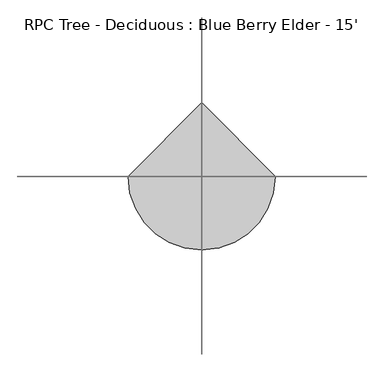
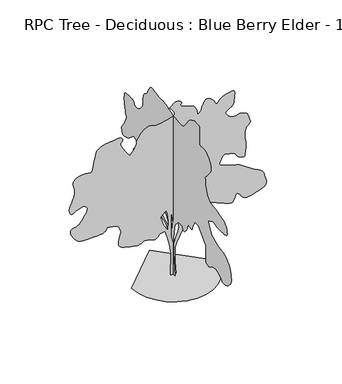
"""IFC4 building model written with IfcOpenShell, lengths in millimetres: geographic element geometry, RPC Tree - Deciduous : Blue Berry Elder - 15'."""

from ifc_helpers import new_model, si_unit, origin, place, context, project, spatial, triangles, source, transform, mapped, element, save


def rpc_tree_deciduous_blue_berry_elder_15_a2d70376(model_context):
    return source(origin(), model_context, "Body", "Tessellation", [
        triangles([(-0.0014919, 59.6430573, 0.0042007), (-0.0014919, -63.4980182, 0.0042007), (-0.0014919, -15.6099892, 574.662743), (-0.0014919, -1.9275415, 923.5625221), (-0.0014919, -22.4510529, 1121.9570257), (-0.0014919, -77.1804997, 1347.7149754), (-0.0014919, -227.6865383, 1498.2227943), (-0.0014919, -385.0338381, 1498.2227943), (-0.0014919, -419.2400351, 1402.4443382), (-0.0014919, -487.6499219, 1409.2870892), (-0.0014919, -562.9051031, 1498.2227943), (-0.0014919, -610.791715, 1593.9986343), (-0.0014919, -638.1577045, 1689.7744743), (-0.0014919, -713.4103786, 1662.4110283), (-0.0014919, -795.5032602, 1655.5682774), (-0.0014919, -870.7558617, 1826.5992622), (-0.0014919, -925.4852972, 1929.2153824), (-0.0014919, -1075.9931162, 1922.3751022), (-0.0014919, -1192.2921947, 1826.5992622), (-0.0014919, -1404.3696568, 1600.8387691), (-0.0014919, -1411.2099369, 1375.0808922), (-0.0014919, -1409.1144253, 1348.2534599), (-0.0014919, -1404.5093285, 1316.2824463), (-0.0014919, -1399.9017609, 1281.557967), (-0.0014919, -1397.8062492, 1246.4730446), (-0.0014919, -1400.7374657, 1213.4249891), (-0.0014919, -1411.2099369, 1184.8042797), (-0.0014919, -1431.7331028, 1163.0034302), (-0.0014919, -1457.4226685, 1147.2477785), (-0.0014919, -1482.2740585, 1135.79746), (-0.0014919, -1507.1254486, 1129.6151339), (-0.0014919, -1532.8150143, 1129.6557564), (-0.0014919, -1560.1810764, 1136.8769726), (-0.0014919, -1590.0565784, 1152.2338114), (-0.0014919, -1623.2873989, 1176.6863886), (-0.0014919, -1664.49375, 1202.6350954), (-0.0014919, -1715.0347057, 1221.7613262), (-0.0014919, -1770.8411831, 1233.9482277), (-0.0014919, -1827.8439537, 1239.0739323), (-0.0014919, -1881.9739346, 1237.0215866), (-0.0014919, -1929.1645134, 1227.6667797), (-0.0014919, -1965.3442818, 1210.8926582), (-0.0014919, -1995.2630951, 1185.7212296), (-0.0014919, -2027.0942917, 1154.4487198), (-0.0014919, -2061.9177475, 1121.8579039), (-0.0014919, -2100.8127571, 1092.7367889), (-0.0014919, -2144.8513481, 1071.8757803), (-0.0014919, -2195.1129604, 1064.0551094), (-0.0014919, -2252.6744179, 1074.0677977), (-0.0014919, -2311.551638, 1100.7352833), (-0.0014919, -2364.3279224, 1137.4535362), (-0.0014919, -2409.9209244, 1180.8748684), (-0.0014919, -2447.2590523, 1227.6464321), (-0.0014919, -2475.2625755, 1274.4181412), (-0.0014919, -2492.8519089, 1317.8368572), (-0.0014919, -2498.9556061, 1354.5577263), (-0.0014919, -2495.0465424, 1394.6871082), (-0.0014919, -2484.4370155, 1446.9019444), (-0.0014919, -2468.7981445, 1505.7005356), (-0.0014919, -2449.8115128, 1565.5759506), (-0.0014919, -2429.1486752, 1621.024165), (-0.0014919, -2408.4858376, 1666.538538), (-0.0014919, -2389.496735, 1696.6146091), (-0.0014919, -2367.4393604, 1721.5473896), (-0.0014919, -2337.0025555, 1752.8198994), (-0.0014919, -2299.0269665, 1786.7288761), (-0.0014919, -2254.3509144, 1819.5584129), (-0.0014919, -2203.8099586, 1847.6000153), (-0.0014919, -2148.2422749, 1867.1453339), (-0.0014919, -2088.4861839, 1874.4858742), (-0.0014919, -2026.3171589, 1879.471907), (-0.0014919, -1963.0710194, 1893.4344269), (-0.0014919, -1898.9284229, 1914.8745426), (-0.0014919, -1834.0668297, 1942.2988861), (-0.0014919, -1768.6668972, 1974.2114731), (-0.0014919, -1702.9062309, 2009.1161739), (-0.0014919, -1636.9678139, 2045.5143883), (-0.0014919, -1493.3027458, 2312.3213585), (-0.0014919, -1712.220488, 2414.9399494), (-0.0014919, -1741.6996479, 2406.2024014), (-0.0014919, -1772.1365982, 2397.8254417), (-0.0014919, -1804.4885479, 2390.1673336), (-0.0014919, -1839.7108166, 2383.5861946), (-0.0014919, -1878.7633747, 2378.4401424), (-0.0014919, -1922.603722, 2375.0899109), (-0.0014919, -1972.187178, 2373.8910015), (-0.0014919, -2028.8316856, 2373.6725555), (-0.0014919, -2090.261657, 2373.8122272), (-0.0014919, -2152.0522167, 2375.5064552), (-0.0014919, -2209.7738388, 2379.9564743), (-0.0014919, -2258.9965611, 2388.3511654), (-0.0014919, -2295.2982697, 2401.8945248), (-0.0014919, -2314.2440609, 2421.7802296), (-0.0014919, -2317.876252, 2453.1136368), (-0.0014919, -2312.2908371, 2496.5351143), (-0.0014919, -2299.1666382, 2546.5297371), (-0.0014919, -2280.1775356, 2597.6091774), (-0.0014919, -2257.0026421, 2644.26912), (-0.0014919, -2231.3130764, 2680.9974014), (-0.0014919, -2204.7853352, 2702.2574409), (-0.0014919, -2178.018655, 2712.9253944), (-0.0014919, -2148.9788578, 2722.1454712), (-0.0014919, -2115.3923904, 2730.9847572), (-0.0014919, -2074.9835197, 2740.5606262), (-0.0014919, -2025.478838, 2751.9398735), (-0.0014919, -1964.605228, 2766.1637146), (-0.0014919, -1890.091753, 2784.3501045), (-0.0014919, -1810.2315113, 2802.4350471), (-0.0014919, -1735.3979977, 2817.522789), (-0.0014919, -1666.4267715, 2832.4579239), (-0.0014919, -1604.1586246, 2850.1870743), (-0.0014919, -1549.4291164, 2873.5298355), (-0.0014919, -1503.0767132, 2905.3557999), (-0.0014919, -1465.9392998, 2948.5613022), (-0.0014919, -1437.478537, 3000.783696), (-0.0014919, -1415.8377068, 3057.3241402), (-0.0014919, -1399.8814133, 3117.4716316), (-0.0014919, -1388.4717899, 3180.4634262), (-0.0014919, -1380.4732956, 3245.6399712), (-0.0014919, -1374.7506798, 3312.238813), (-0.0014919, -1370.1634598, 3379.5489487), (-0.0014919, -1421.161655, 3432.3047401), (-0.0014919, -1470.3080738, 3484.9335045), (-0.0014919, -1515.7412018, 3537.3337944), (-0.0014919, -1555.6115879, 3589.3785828), (-0.0014919, -1588.0626595, 3640.9149719), (-0.0014919, -1611.2401691, 3691.8929649), (-0.0014919, -1623.2873989, 3742.1340843), (-0.0014919, -1619.2183159, 3797.684182), (-0.0014919, -1597.4378139, 3860.6506874), (-0.0014919, -1561.1766552, 3925.0397804), (-0.0014919, -1513.6685085, 3984.9076378), (-0.0014919, -1458.1415199, 4034.2345688), (-0.0014919, -1397.8265968, 4067.0258812), (-0.0014919, -1335.9572628, 4077.3383331), (-0.0014919, -1278.5939037, 4074.2649742), (-0.0014919, -1229.7292992, 4071.8773293), (-0.0014919, -1189.4804478, 4071.7755913), (-0.0014919, -1157.966601, 4075.509375), (-0.0014919, -1135.3097717, 4084.6280045), (-0.0014919, -1121.6268133, 4100.6808037), (-0.0014919, -1117.0395206, 4125.2426765), (-0.0014919, -1118.7743711, 4171.0390091), (-0.0014919, -1122.5437632, 4241.9559013), (-0.0014919, -1126.1936857, 4326.2838936), (-0.0014919, -1127.5704185, 4412.288237), (-0.0014919, -1124.5173346, 4488.2344734), (-0.0014919, -1114.885655, 4542.4125618), (-0.0014919, -1096.5163548, 4563.0627548), (-0.0014919, -1069.6304232, 4564.4597626), (-0.0014919, -1037.2377783, 4567.5331215), (-0.0014919, -1001.3780485, 4570.6067711), (-0.0014919, -964.0806158, 4572.0037788), (-0.0014919, -927.380167, 4570.0477936), (-0.0014919, -893.3136417, 4563.0627548), (-0.0014919, -863.9156542, 4549.3976006), (-0.0014919, -835.993376, 4533.1416161), (-0.0014919, -805.556571, 4518.3587975), (-0.0014919, -773.4433422, 4503.0678703), (-0.0014919, -740.4944086, 4485.3895889), (-0.0014919, -707.545475, 4463.4185463), (-0.0014919, -675.4347897, 4435.2246277), (-0.0014919, -644.9979847, 4398.877137), (-0.0014919, -614.4824055, 4355.0112099), (-0.0014919, -581.8128516, 4307.6911331), (-0.0014919, -547.3475862, 4260.1167114), (-0.0014919, -511.4446541, 4215.5397812), (-0.0014919, -474.4672963, 4177.1857269), (-0.0014919, -436.7711234, 4148.2805145), (-0.0014919, -398.7168328, 4132.075399), (-0.0014919, -359.7633602, 4126.0048393), (-0.0014919, -319.1360072, 4124.6078316), (-0.0014919, -276.8322849, 4126.6905533), (-0.0014919, -232.8521387, 4131.0338928), (-0.0014919, -187.1978941, 4136.4696075), (-0.0014919, -139.8680069, 4141.7780045), (-0.0014919, -90.8629858, 4145.7658424), (-0.0014919, -33.0220578, 4153.2081207), (-0.0014919, 35.9481419, 4167.7368851), (-0.0014919, 108.7479043, 4186.3296455), (-0.0014919, 178.0769938, 4205.989492), (-0.0014919, 236.6359921, 4223.7439316), (-0.0014919, 277.1243819, 4236.5963448), (-0.0014919, 292.2424816, 4241.523951), (-0.0014919, 300.5609782, 4244.1147812), (-0.0014919, 323.5962728, 4250.5411331), (-0.0014919, 358.4806623, 4258.7705727), (-0.0014919, 402.3388501, 4266.7462486), (-0.0014919, 452.3032422, 4272.4357269), (-0.0014919, 505.495962, 4273.8327347), (-0.0014919, 559.0493792, 4268.9051285), (-0.0014919, 618.0663437, 4267.9400711), (-0.0014919, 686.0596498, 4278.836499), (-0.0014919, 757.7613779, 4295.8293571), (-0.0014919, 827.9085497, 4313.1774261), (-0.0014919, 891.2359343, 4325.1409401), (-0.0014919, 942.4728504, 4325.9789703), (-0.0014919, 976.3615522, 4309.9517509), (-0.0014919, 999.7371603, 4282.3926773), (-0.0014919, 1022.6327831, 4252.7761711), (-0.0014919, 1044.5733044, 4221.6359207), (-0.0014919, 1065.0761953, 4189.4032951), (-0.0014919, 1083.6639416, 4156.5608231), (-0.0014919, 1099.8614994, 4123.6171944), (-0.0014919, 1113.1837967, 4091.0287766), (-0.0014919, 1129.0994677, 4063.2159393), (-0.0014919, 1151.7182178, 4042.0067688), (-0.0014919, 1178.5228317, 4023.896537), (-0.0014919, 1207.0064129, 4005.4308037), (-0.0014919, 1234.6492023, 3983.1295486), (-0.0014919, 1258.9419056, 3953.5130424), (-0.0014919, 1277.3720306, 3913.1524246), (-0.0014919, 1288.5608826, 3878.2275215), (-0.0014919, 1294.0066257, 3861.6157448), (-0.0014919, 1295.50261, 3854.8086021), (-0.0014919, 1294.8448013, 3849.3223091), (-0.0014919, 1293.8262589, 3836.6730812), (-0.0014919, 1294.245274, 3808.3265556), (-0.0014919, 1297.8953419, 3755.7995293), (-0.0014919, 1304.3392799, 3695.8046448), (-0.0014919, 1312.5765678, 3648.6365936), (-0.0014919, 1323.5645599, 3611.1208603), (-0.0014919, 1338.2635174, 3580.2090843), (-0.0014919, 1357.6310852, 3552.7770378), (-0.0014919, 1382.622147, 3525.6752037), (-0.0014919, 1414.1969639, 3495.8555122), (-0.0014919, 1450.0566936, 3466.1628479), (-0.0014919, 1486.6377457, 3441.8806091), (-0.0014919, 1522.9750626, 3423.3131378), (-0.0014919, 1558.118557, 3410.8670952), (-0.0014919, 1591.1081131, 3404.8979828), (-0.0014919, 1620.9860859, 3405.7363037), (-0.0014919, 1646.795121, 3413.7628487), (-0.0014919, 1665.9440975, 3429.5107246), (-0.0014919, 1679.3451691, 3450.9992386), (-0.0014919, 1691.3136246, 3474.7736595), (-0.0014919, 1706.1523991, 3497.354258), (-0.0014919, 1728.1716946, 3515.2613045), (-0.0014919, 1761.6793877, 3525.0403587), (-0.0014919, 1810.9833549, 3523.2114006), (-0.0014919, 1870.0002468, 3519.655513), (-0.0014919, 1927.9427856, 3522.4495285), (-0.0014919, 1982.0524189, 3525.3702805), (-0.0014919, 2029.5835293, 3522.1698944), (-0.0014919, 2067.7775642, 3506.6504929), (-0.0014919, 2093.8862904, 3472.5891998), (-0.0014919, 2105.1536259, 3413.7628487), (-0.0014919, 2107.5870529, 3355.0888138), (-0.0014919, 2108.7045719, 3318.9189285), (-0.0014919, 2108.0264156, 3295.0939293), (-0.0014919, 2105.0749969, 3273.4275192), (-0.0014919, 2099.3701126, 3243.7095657), (-0.0014919, 2090.4343208, 3195.8305115), (-0.0014919, 2077.7901798, 3119.5796425), (-0.0014919, 2061.2548519, 3041.6777115), (-0.0014919, 2043.5255562, 2988.8966309), (-0.0014919, 2028.4253151, 2951.2030014), (-0.0014919, 2019.7893597, 2918.5384254), (-0.0014919, 2021.4453632, 2880.844796), (-0.0014919, 2037.2212898, 2828.0637154), (-0.0014919, 2070.9474289, 2750.1617844), (-0.0014919, 2114.4501514, 2668.4752007), (-0.0014919, 2155.0774681, 2607.7440239), (-0.0014919, 2189.9618214, 2562.9383286), (-0.0014919, 2216.2279507, 2529.0063881), (-0.0014919, 2231.0082985, 2500.9418221), (-0.0014919, 2231.4273136, 2473.7181931), (-0.0014919, 2214.6124969, 2442.3032501), (-0.0014919, 2195.0062809, 2409.7735497), (-0.0014919, 2184.256937, 2383.1061367), (-0.0014919, 2175.300943, 2363.1416576), (-0.0014919, 2161.0794273, 2350.7159626), (-0.0014919, 2134.5339546, 2346.6672272), (-0.0014919, 2088.6004211, 2351.8336269), (-0.0014919, 2016.218066, 2367.0507214), (-0.0014919, 1937.2366951, 2396.3496597), (-0.0014919, 1873.5715405, 2438.0946407), (-0.0014919, 1821.2754593, 2484.6274109), (-0.0014919, 1776.3986927, 2528.2875366), (-0.0014919, 1734.9940979, 2561.4142937), (-0.0014919, 1693.1069744, 2576.3494286), (-0.0014919, 1646.795121, 2565.45271), (-0.0014919, 1602.1392712, 2539.6566101), (-0.0014919, 1566.8155552, 2514.9450371), (-0.0014919, 1539.2717422, 2491.129921), (-0.0014919, 1517.9509506, 2468.0336563), (-0.0014919, 1501.2961533, 2445.4757309), (-0.0014919, 1487.7527939, 2423.2762138), (-0.0014919, 1475.7666069, 2401.2569183), (-0.0014919, 1494.8139908, 2382.2881634), (-0.0014919, 1513.8006226, 2363.8605091), (-0.0014919, 1532.6702557, 2346.5072079), (-0.0014919, 1551.3570511, 2330.7719765), (-0.0014919, 1569.8076691, 2317.1879219), (-0.0014919, 1587.9584507, 2306.2990517), (-0.0014919, 1605.7486439, 2298.6383274), (-0.0014919, 1624.7173988, 2295.1686264), (-0.0014919, 1645.2405647, 2294.3304508), (-0.0014919, 1665.5250824, 2292.895364), (-0.0014919, 1683.7749859, 2287.6299877), (-0.0014919, 1698.1945999, 2275.3032692), (-0.0014919, 1706.9905746, 2252.6845917), (-0.0014919, 1708.3672348, 2216.5455185), (-0.0014919, 1703.8180939, 2176.2559719), (-0.0014919, 1696.2794552, 2141.3512711), (-0.0014919, 1686.106675, 2108.8417728), (-0.0014919, 1673.6606323, 2075.7328926), (-0.0014919, 1659.3020611, 2039.0323711), (-0.0014919, 1643.3838467, 1995.7533268), (-0.0014919, 1626.2718098, 1942.8984135), (-0.0014919, 1608.601086, 1883.4013184), (-0.0014919, 1592.1266556, 1823.7848991), (-0.0014919, 1578.8829872, 1766.4443584), (-0.0014919, 1570.9048405, 1713.7673412), (-0.0014919, 1570.2266842, 1668.1539917), (-0.0014919, 1578.8829872, 1631.9944256), (-0.0014919, 1598.9083637, 1607.6815201), (-0.0014919, 1624.6970512, 1591.4839622), (-0.0014919, 1649.4087696, 1577.8035473), (-0.0014919, 1673.2237404, 1566.2135571), (-0.0014919, 1696.320005, 1556.3023888), (-0.0014919, 1718.8777851, 1547.6460857), (-0.0014919, 1741.0774475, 1539.8279583), (-0.0014919, 1763.096743, 1532.4263752), (-0.0014919, 1786.3707584, 1542.3400143), (-0.0014919, 1808.5702755, 1550.1581417), (-0.0014919, 1828.6159996, 1553.787862), (-0.0014919, 1845.4283455, 1551.135989), (-0.0014919, 1857.9352856, 1540.1073017), (-0.0014919, 1865.0549091, 1518.6062885), (-0.0014919, 1865.7127178, 1484.5397633), (-0.0014919, 1859.7895329, 1448.2787498), (-0.0014919, 1848.4813568, 1420.635815), (-0.0014919, 1832.6850826, 1400.1710758), (-0.0014919, 1813.2973125, 1385.4517708), (-0.0014919, 1791.2171196, 1375.040197), (-0.0014919, 1767.3435768, 1367.5015583), (-0.0014919, 1742.570961, 1361.3978611), (-0.0014919, 1730.8234222, 1353.9581989), (-0.0014919, 1718.9565594, 1345.8607281), (-0.0014919, 1706.8509029, 1336.4474945), (-0.0014919, 1694.3845127, 1325.0580734), (-0.0014919, 1681.4406807, 1311.0372723), (-0.0014919, 1667.8974667, 1293.7246662), (-0.0014919, 1653.6378719, 1272.4623013), (-0.0014919, 1633.9909607, 1249.8053993), (-0.0014919, 1605.3701786, 1228.5837296), (-0.0014919, 1569.2691845, 1208.558353), (-0.0014919, 1527.1838173, 1189.4905489), (-0.0014919, 1480.6129681, 1171.1415962), (-0.0014919, 1431.0498596, 1153.270158), (-0.0014919, 1379.9907669, 1135.6399841), (-0.0014919, 1215.8024603, 1231.4158241), (-0.0014919, 1051.6141537, 1108.2739946), (-0.0014919, 1029.6533575, 1105.4215525), (-0.0014919, 1007.8727829, 1103.0492409), (-0.0014919, 986.4529421, 1101.6318855), (-0.0014919, 965.5690424, 1101.6522331), (-0.0014919, 945.4065376, 1103.5877254), (-0.0014919, 926.1380917, 1107.915877), (-0.0014919, 907.9491583, 1115.1167456), (-0.0014919, 891.075915, 1124.6493759), (-0.0014919, 875.1577005, 1135.2589754), (-0.0014919, 859.4808231, 1146.3486328), (-0.0014919, 843.3263586, 1157.3188934), (-0.0014919, 825.97313, 1167.5703753), (-0.0014919, 806.7071548, 1176.5060944), (-0.0014919, 784.8072561, 1183.5266687), (-0.0014919, 760.1565805, 1188.9927595), (-0.0014919, 733.3493505, 1193.7399988), (-0.0014919, 704.7489887, 1197.8877834), (-0.0014919, 674.710924, 1201.5581263), (-0.0014919, 643.59589, 1204.8677353), (-0.0014919, 611.7645481, 1207.9411669), (-0.0014919, 579.5725814, 1210.8926582), (-0.0014919, 367.4951194, 1149.3204718), (-0.0014919, 189.6253804, 1019.3383621), (-0.0014919, 93.8490136, 861.9928791), (-0.0014919, 45.9605758, 560.9797846), (-0.0013978, 66.484046, 1115.1167456), (-0.0013978, 169.1019057, 1334.0344151), (-0.0013978, 4.9135321, 1402.4443382), (-0.0014104, 312.7656838, 1190.3694197), (-0.0014104, 476.9539541, 1299.8282181), (-0.0014104, 606.9360274, 1306.6684982), (-0.0014104, 716.3948622, 1368.2381413), (-0.0014104, 710.4918795, 1371.410622), (-0.0014104, 704.3476324, 1376.0181896), (-0.0014104, 697.7284143, 1383.4984016), (-0.0014104, 690.3878014, 1395.2840195), (-0.0014104, 682.089616, 1412.8176876), (-0.0014104, 672.5976082, 1437.529406), (-0.0014104, 661.6654266, 1470.8567322), (-0.0014104, 652.9303493, 1503.7853909), (-0.0014104, 649.5801178, 1527.3819157), (-0.0014104, 650.7155136, 1543.1985374), (-0.0014104, 655.442478, 1552.7921379), (-0.0014104, 662.864336, 1557.7172733), (-0.0014104, 672.0769278, 1559.5332962), (-0.0014104, 682.1912086, 1559.7924374), (-0.0014104, 689.0314161, 1641.8852463), (-0.0014104, 606.9360274, 1696.6146091), (-0.0014104, 429.0673059, 1546.1094063), (-0.0014104, 305.9254764, 1402.4443382), (-0.0014104, 223.8310687, 1286.1453323), (-0.0014104, 141.7369426, 1101.4337872), (67.7022311, 0.0002671, 0.0), (-69.1215849, 0.0002671, 0.0), (-62.2805962, 0.0002309, 560.9772411), (-96.4865524, 0.0002173, 807.2583567), (-144.3744815, 0.0002037, 1012.4930677), (-205.9448967, 0.0001946, 1197.2045403), (-329.0852182, 0.0001946, 1183.5241253), (-349.6693906, 0.0001946, 1154.5020596), (-370.6116806, 0.0001992, 1127.2782852), (-392.2728221, 0.0001992, 1103.6436087), (-415.0109327, 0.0001992, 1085.3936325), (-439.1841302, 0.0002037, 1074.3243227), (-465.1505685, 0.0002037, 1072.2288111), (-493.2734885, 0.0001992, 1080.9054617), (-523.1921565, 0.0001992, 1093.9686905), (-554.1877936, 0.0001992, 1104.1617456), (-586.0800694, 0.0001992, 1111.9595255), (-618.6886168, 0.0001992, 1117.8447041), (-651.8381922, 0.0001992, 1122.2922523), (-685.3458853, 0.0001992, 1125.7822283), (-719.0339453, 0.0001992, 1128.7946898), (-746.9764984, 0.0001992, 1112.8383963), (-775.4575361, 0.0001992, 1097.8981018), (-805.0180864, 0.0001992, 1084.9948923), (-836.191547, 0.0001992, 1075.1422234), (-869.5188732, 0.0002037, 1069.3586374), (-905.5412384, 0.0002037, 1068.6601336), (-944.7918222, 0.0002037, 1074.0652542), (-995.5334925, 0.0001992, 1083.856953), (-1060.8724548, 0.0001992, 1096.2826481), (-1133.6334206, 0.0001992, 1112.2999117), (-1206.6330345, 0.0001992, 1132.8637728), (-1272.690921, 0.0001946, 1158.9318037), (-1324.6262684, 0.0001946, 1191.4615768), (-1355.2613171, 0.0001901, 1231.4107372), (-1365.1546085, 0.0001901, 1279.0206219), (-1362.3630638, 0.0001856, 1331.6544731), (-1350.9534405, 0.0001811, 1385.9672916), (-1334.997147, 0.0001811, 1438.6012882), (-1318.5632664, 0.0001765, 1486.2110275), (-1305.7185562, 0.0001765, 1525.4413364), (-1300.5318089, 0.000172, 1552.9470703), (-1302.9068092, 0.000172, 1576.4623501), (-1309.4676006, 0.000172, 1604.5243), (-1319.3812397, 0.0001675, 1634.9815979), (-1331.8069347, 0.0001675, 1665.6773987), (-1345.9089809, 0.000163, 1694.4582001), (-1360.8467319, 0.000163, 1719.1699184), (-1375.7869537, 0.000163, 1737.6586155), (-1395.4313942, 0.000163, 1750.9224861), (-1424.0546471, 0.0001584, 1761.6716846), (-1460.1531704, 0.0001584, 1770.328133), (-1502.2385376, 0.0001584, 1777.3079395), (-1548.8093868, 0.0001584, 1783.0331715), (-1598.3724953, 0.0001584, 1787.9200825), (-1649.431588, 0.0001584, 1792.3879784), (-1657.3716557, 0.0001584, 1766.1802757), (-1668.9591751, 0.000163, 1741.0495422), (-1687.8465397, 0.000163, 1718.0726017), (-1717.6865788, 0.000163, 1698.3265686), (-1762.1238373, 0.000163, 1682.8885574), (-1824.8111446, 0.0001675, 1672.8377174), (-1909.398278, 0.0001675, 1669.2462215), (-2003.1193016, 0.0001675, 1666.9119164), (-2090.3809811, 0.0001675, 1662.3043488), (-2170.5789928, 0.0001675, 1659.0150146), (-2243.1190418, 0.0001675, 1660.6304684), (-2307.4039261, 0.0001675, 1670.7422058), (-2362.8293221, 0.000163, 1692.9418682), (-2408.80326, 0.000163, 1730.8183353), (-2450.3908379, 0.0001584, 1780.5998898), (-2490.1799789, 0.0001584, 1834.2117336), (-2523.8680389, 0.0001539, 1888.783548), (-2547.1392929, 0.0001494, 1941.4378922), (-2555.6992355, 0.0001449, 1989.3067726), (-2545.2344673, 0.0001449, 2029.5149288), (-2511.4219963, 0.0001449, 2059.1923325), (-2467.3223625, 0.0001403, 2077.8410488), (-2428.3689262, 0.0001403, 2089.431039), (-2393.8453068, 0.0001403, 2097.7876511), (-2363.0298912, 0.0001403, 2106.7437904), (-2335.2067348, 0.0001403, 2120.1269852), (-2309.6568409, 0.0001358, 2141.7653446), (-2285.6615032, 0.0001358, 2175.4939545), (-2257.2616379, 0.0001313, 2219.9110107), (-2222.6364258, 0.0001313, 2269.4739738), (-2187.2922169, 0.0001267, 2321.7904026), (-2156.7360878, 0.0001222, 2374.464949), (-2136.4719177, 0.0001222, 2425.1076427), (-2132.0040218, 0.0001177, 2471.3203743), (-2148.8391861, 0.0001177, 2510.7107025), (-2179.7535782, 0.0001132, 2538.5136566), (-2213.5406147, 0.0001132, 2553.0322472), (-2249.7203831, 0.0001132, 2556.4866875), (-2287.8154415, 0.0001132, 2551.0765526), (-2327.3479122, 0.0001132, 2539.0342644), (-2367.8355572, 0.0001132, 2522.5573631), (-2408.80326, 0.0001177, 2503.8704224), (-2437.9625267, 0.0001177, 2487.9929031), (-2466.1666191, 0.0001177, 2473.6141296), (-2492.453096, 0.0001177, 2462.2247086), (-2515.8670738, 0.0001177, 2455.3233856), (-2535.4554131, 0.0001177, 2454.4065811), (-2550.2635208, 0.0001177, 2460.9672272), (-2559.3059921, 0.0001177, 2476.5046509), (-2566.1387146, 0.0001177, 2495.7526039), (-2573.6824402, 0.0001177, 2514.0433479), (-2580.1340813, 0.0001132, 2533.7688881), (-2583.7155487, 0.0001132, 2557.3247177), (-2582.6487534, 0.0001132, 2587.0935402), (-2575.1047371, 0.0001086, 2625.4984634), (-2559.3059921, 0.0001041, 2674.9015526), (-2538.1680382, 0.0001041, 2727.6064751), (-2516.667025, 9.96e-05, 2775.7904526), (-2496.1235115, 9.96e-05, 2821.5612053), (-2477.8534058, 9.51e-05, 2867.0781944), (-2463.1746506, 9.05e-05, 2914.5505875), (-2453.4005379, 9.05e-05, 2966.0619781), (-2449.8498825, 8.6e-05, 3023.7962448), (-2453.8603935, 8.15e-05, 3079.1681557), (-2463.4920731, 8.15e-05, 3124.1261673), (-2475.1608376, 7.7e-05, 3161.6674805), (-2485.2727203, 7.7e-05, 3194.7637161), (-2490.240731, 7.24e-05, 3226.4376549), (-2486.4688683, 7.24e-05, 3259.6609177), (-2470.3753738, 6.79e-05, 3297.4559944), (-2440.0783859, 6.79e-05, 3333.6511688), (-2398.8922371, 6.34e-05, 3360.8800301), (-2351.003009, 6.34e-05, 3380.2093735), (-2300.601725, 6.34e-05, 3392.7059944), (-2251.8769375, 6.34e-05, 3399.4625587), (-2209.0144375, 6.34e-05, 3401.5708603), (-2176.2051029, 6.34e-05, 3400.0721146), (-2148.061908, 6.34e-05, 3394.4587944), (-2117.7647747, 6.34e-05, 3386.2290642), (-2087.3483173, 6.34e-05, 3379.4219215), (-2058.8468594, 6.34e-05, 3378.1263611), (-2034.2926895, 6.34e-05, 3386.4069603), (-2015.7253635, 6.34e-05, 3408.3271339), (-2005.174118, 5.88e-05, 3447.9511688), (-1996.2586739, 5.43e-05, 3505.228196), (-1982.4359711, 5.43e-05, 3573.6559959), (-1965.5043011, 4.98e-05, 3647.5697983), (-1947.2543976, 4.53e-05, 3721.3568642), (-1929.4820812, 4.07e-05, 3789.4035828), (-1913.985498, 3.62e-05, 3846.0963432), (-1902.5555271, 3.17e-05, 3885.7968269), (-1882.1516853, 3.17e-05, 3914.5241432), (-1842.3625443, 3.17e-05, 3941.473661), (-1788.9284512, 2.72e-05, 3965.6797417), (-1727.5976017, 2.72e-05, 3986.1523293), (-1664.1128139, 2.72e-05, 4001.9763634), (-1604.2170513, 2.72e-05, 4012.1617882), (-1553.655748, 2.72e-05, 4015.7685448), (-1506.505719, 2.72e-05, 4019.2738541), (-1455.4059311, 2.72e-05, 4027.0969231), (-1403.9480255, 2.72e-05, 4035.1487572), (-1355.7210274, 2.26e-05, 4039.3906494), (-1314.3139618, 2.72e-05, 4035.7077347), (-1283.3207954, 2.72e-05, 4020.0865952), (-1266.3256119, 2.72e-05, 3988.4126564), (-1265.9090675, 3.17e-05, 3953.5130424), (-1277.2170982, 3.17e-05, 3927.1225021), (-1292.7136814, 3.17e-05, 3903.5003975), (-1304.8625038, 3.62e-05, 3876.8813828), (-1306.1173691, 3.62e-05, 3841.4989494), (-1288.9442894, 4.07e-05, 3791.6642006), (-1245.8049168, 4.53e-05, 3721.6109184), (-1194.5655298, 4.98e-05, 3646.731768), (-1155.891437, 4.98e-05, 3586.6860146), (-1126.4324793, 5.43e-05, 3542.0835045), (-1102.8384253, 5.43e-05, 3513.5340843), (-1081.7563545, 5.88e-05, 3501.5958595), (-1059.8361809, 5.43e-05, 3506.9045471), (-1033.7274548, 5.43e-05, 3530.0441231), (-1006.0846653, 5.43e-05, 3563.4705711), (-981.7894913, 4.98e-05, 3598.9288719), (-960.8472376, 4.98e-05, 3635.9620766), (-943.2576862, 4.53e-05, 3674.0620766), (-929.0158957, 4.53e-05, 3712.7463432), (-918.1268801, 4.07e-05, 3751.557637), (-910.5856253, 4.07e-05, 3790.0131386), (-896.7832701, 3.62e-05, 3834.3363052), (-868.8610645, 3.17e-05, 3887.3714401), (-829.4503887, 3.17e-05, 3943.65783), (-781.1826954, 2.72e-05, 3997.6838928), (-726.6920534, 2.26e-05, 4043.9118851), (-668.6123863, 2.26e-05, 4076.8558044), (-609.5750742, 2.26e-05, 4091.0287766), (-561.6655712, 2.26e-05, 4089.1745293), (-529.5548495, 2.26e-05, 4080.3608231), (-504.7415749, 2.26e-05, 4068.5752052), (-478.734514, 2.26e-05, 4057.7549355), (-443.0322238, 2.26e-05, 4051.836692), (-389.1410002, 2.26e-05, 4054.7577347), (-308.5619797, 2.26e-05, 4070.5056107), (-218.1912603, 2.26e-05, 4091.0034874), (-140.9838273, 2.26e-05, 4107.2086029), (-77.5383903, 1.81e-05, 4121.4836037), (-28.4536116, 1.81e-05, 4136.2408424), (5.6723577, 1.81e-05, 4153.8685455), (24.2412211, 1.81e-05, 4176.7540672), (26.6545277, 1.36e-05, 4207.310051), (18.5968788, 1.36e-05, 4240.5080246), (6.5899843, 9.1e-06, 4270.098951), (-8.707838, 9.1e-06, 4296.7182564), (-26.6385244, 9.1e-06, 4320.924337), (-46.5435071, 4.5e-06, 4343.3526192), (-67.764968, 4.5e-06, 4364.5617897), (-89.6448007, 4.5e-06, 4385.1864029), (-61.8612404, 4.5e-06, 4411.3740486), (-34.4965295, 0.0, 4436.3675812), (-7.9696625, 0.0, 4458.9734688), (17.3007665, 0.0, 4477.9728905), (40.8958095, 0.0, 4492.1967316), (62.3966728, -4.5e-06, 4500.4264618), (81.3844583, -4.5e-06, 4501.4932571), (101.1299282, -4.5e-06, 4497.6833153), (123.747879, 0.0, 4491.9682571), (147.0833914, 0.0, 4484.0687393), (168.9832901, 0.0, 4473.8071564), (187.292892, 0.0, 4460.9038742), (199.8582769, 0.0, 4445.1304184), (204.5255429, 0.0, 4426.2330254), (200.2771285, 4.5e-06, 4409.087851), (190.6436686, 4.5e-06, 4397.0737587), (180.2923927, 4.5e-06, 4387.8281021), (173.8900582, 4.5e-06, 4378.9382378), (176.103931, 4.5e-06, 4367.9906502), (191.6012409, 4.5e-06, 4352.6491447), (225.0492538, 9.1e-06, 4330.4749168), (270.045399, 9.1e-06, 4307.8943184), (316.1184952, 9.1e-06, 4291.4095688), (361.8334373, 9.1e-06, 4278.7603409), (405.7526316, 9.1e-06, 4267.6860168), (446.4409184, 1.36e-05, 4255.8751099), (482.4607038, 1.36e-05, 4241.0667114), (512.3793717, 1.36e-05, 4221.0007851), (536.1741039, 1.36e-05, 4195.1436424), (555.3003347, 1.81e-05, 4164.9937386), (570.5378131, 1.81e-05, 4131.2623672), (582.6637808, 2.26e-05, 4094.6355331), (592.4580231, 2.26e-05, 4055.8498192), (600.6952383, 2.72e-05, 4015.6415176), (608.1552117, 2.72e-05, 3974.722213), (703.9310881, 2.26e-05, 4063.647599), (703.2935543, 2.26e-05, 4067.2543556), (702.1759626, 2.26e-05, 4077.3127533), (701.7771498, 2.26e-05, 4092.7307076), (703.2935543, 2.26e-05, 4112.4920013), (707.9213968, 1.81e-05, 4135.4533905), (716.8571886, 1.81e-05, 4160.59953), (731.2970776, 1.81e-05, 4186.7868851), (747.8502823, 1.36e-05, 4214.0666153), (763.2096645, 1.36e-05, 4241.5748199), (778.6859001, 9.1e-06, 4267.025592), (795.599766, 9.1e-06, 4288.2091827), (815.2644814, 9.1e-06, 4302.7888161), (838.9982071, 9.1e-06, 4308.5038742), (868.119322, 9.1e-06, 4303.0937393), (898.3758327, 9.1e-06, 4289.9872719), (925.0433184, 9.1e-06, 4274.3408432), (948.7186901, 1.36e-05, 4256.6116928), (969.9988592, 1.36e-05, 4237.2059006), (989.4857512, 1.36e-05, 4216.5304184), (1007.7737337, 1.36e-05, 4195.0419044), (1025.4674212, 1.81e-05, 4173.1217308), (1029.993671, 1.81e-05, 4151.4047424), (1035.2997425, 1.81e-05, 4131.2879471), (1042.1602976, 1.81e-05, 4114.4224068), (1051.3550852, 2.26e-05, 4102.3827347), (1063.6613834, 2.26e-05, 4096.8199928), (1079.8564705, 2.26e-05, 4099.3346649), (1100.7200226, 2.26e-05, 4111.5522331), (1123.5978413, 1.81e-05, 4132.811982), (1146.3537197, 1.81e-05, 4159.3295494), (1170.5472284, 1.81e-05, 4188.0062874), (1197.732851, 1.36e-05, 4215.7429665), (1229.4650711, 1.36e-05, 4239.3903603), (1267.3009884, 1.36e-05, 4255.8751099), (1312.7950138, 1.36e-05, 4262.0471169), (1361.8805351, 9.1e-06, 4267.2796463), (1408.0932667, 9.1e-06, 4278.7350517), (1449.398885, 9.1e-06, 4290.06343), (1483.7651012, 9.1e-06, 4294.9148781), (1509.1549759, 9.1e-06, 4286.9900711), (1523.5363655, 1.36e-05, 4259.888237), (1524.8724758, 1.36e-05, 4207.310051), (1519.9652172, 1.81e-05, 4142.8703796), (1515.7766647, 2.26e-05, 4084.5009773), (1510.5112885, 2.72e-05, 4032.4817688), (1502.3755932, 2.72e-05, 3987.0412285), (1489.5689621, 3.17e-05, 3948.43312), (1470.3029869, 3.17e-05, 3916.8862083), (1442.7795216, 3.17e-05, 3892.6292587), (1408.3320602, 3.62e-05, 3872.7156487), (1372.4519829, 3.62e-05, 3853.18312), (1339.5615486, 3.62e-05, 3832.6852432), (1314.0928997, 3.62e-05, 3809.9014595), (1300.4709114, 4.07e-05, 3783.5362083), (1303.1226391, 4.07e-05, 3752.243351), (1326.4778996, 4.53e-05, 3714.7529068), (1361.2023788, 4.53e-05, 3678.8882355), (1394.8497437, 4.98e-05, 3652.3703773), (1427.1814911, 4.98e-05, 3633.6253006), (1457.9560661, 4.98e-05, 3621.1030998), (1486.937582, 4.98e-05, 3613.2291618), (1513.8818676, 4.98e-05, 3608.4791611), (1538.5553616, 4.98e-05, 3605.3043549), (1559.4774857, 4.98e-05, 3606.8028099), (1576.9297634, 4.98e-05, 3614.7531967), (1593.3026012, 4.98e-05, 3625.5734665), (1610.9962887, 4.98e-05, 3635.7080223), (1632.3958546, 4.98e-05, 3641.4992386), (1659.9014431, 4.98e-05, 3639.4165169), (1695.9009899, 4.98e-05, 3625.8275208), (1734.0771481, 4.98e-05, 3609.6729836), (1766.7466656, 4.98e-05, 3599.6145859), (1794.2701309, 4.98e-05, 3591.7153587), (1817.0082779, 4.98e-05, 3582.0124626), (1835.316608, 5.43e-05, 3566.5945084), (1849.558326, 5.43e-05, 3541.4486595), (1860.0892239, 5.88e-05, 3502.6882347), (1872.6545906, 5.88e-05, 3459.6350487), (1889.4085098, 6.34e-05, 3423.0590836), (1905.3241081, 6.34e-05, 3391.0296432), (1915.3774189, 6.34e-05, 3361.6419022), (1914.5392433, 6.79e-05, 3332.939875), (1897.7853241, 6.79e-05, 3303.0693146), (1860.0892239, 7.24e-05, 3270.0748169), (1819.3424377, 7.24e-05, 3225.0150673), (1794.6308647, 7.7e-05, 3164.2835999), (1782.7233067, 8.15e-05, 3093.9765541), (1780.3890015, 8.6e-05, 3020.2147774), (1784.397187, 9.05e-05, 2949.0694107), (1791.5192814, 9.51e-05, 2886.6615921), (1798.5195808, 9.51e-05, 2839.0871704), (1802.5886639, 9.96e-05, 2800.3776146), (1803.4268394, 9.96e-05, 2760.5756836), (1801.5701214, 0.0001041, 2719.8848534), (1797.5619358, 0.0001041, 2678.48302), (1791.9384418, 0.0001086, 2636.5474983), (1785.2353626, 0.0001086, 2594.2311859), (1777.9964149, 0.0001132, 2551.7622665), (1779.0935863, 0.0001132, 2530.0377205), (1777.9760674, 0.0001177, 2509.9334244), (1772.4312023, 0.0001177, 2493.0603264), (1760.2443008, 0.0001177, 2481.0334442), (1739.2028526, 0.0001177, 2475.4680862), (1707.0896965, 0.0001177, 2477.9801422), (1661.6947929, 0.0001177, 2490.1875366), (1618.3547058, 0.0001177, 2511.8867935), (1589.7339237, 0.0001132, 2539.8115425), (1569.6094254, 0.0001132, 2570.9645828), (1551.7583347, 0.0001086, 2602.3591782), (1529.9574852, 0.0001086, 2631.0103363), (1497.9864716, 0.0001086, 2653.895858), (1449.6198017, 0.0001086, 2668.0688301), (1395.7870411, 0.0001041, 2678.0257805), (1350.6918285, 0.0001041, 2688.3635216), (1313.0159306, 0.0001041, 2696.0598541), (1281.4411137, 0.0001041, 2698.1425758), (1254.6568474, 0.0001041, 2691.5894875), (1231.339666, 0.0001041, 2673.4536758), (1210.1788937, 0.0001086, 2640.6876526), (1189.6938068, 0.0001086, 2600.6063782), (1171.1263355, 0.0001132, 2562.9127487), (1157.2249311, 0.0001132, 2528.3229996), (1150.7428413, 0.0001177, 2497.566156), (1154.4309156, 0.0001177, 2471.3584534), (1171.0450905, 0.0001177, 2450.416127), (1203.3361427, 0.0001222, 2435.4580284), (1238.8200233, 0.0001222, 2424.8078064), (1266.0436523, 0.0001222, 2415.5926712), (1289.3202839, 0.0001222, 2406.7382698), (1312.9550331, 0.0001222, 2397.1625462), (1341.2582474, 0.0001222, 2385.7959435), (1378.5353325, 0.0001222, 2371.5542255), (1429.0966358, 0.0001267, 2353.3652195), (1483.0867996, 0.0001267, 2336.5300552), (1529.2996765, 0.0001267, 2325.0823528), (1570.0082382, 0.0001267, 2316.0272369), (1607.4860378, 0.0001267, 2306.3725937), (1644.0035763, 0.0001267, 2293.1290707), (1681.8394936, 0.0001313, 2273.3044086), (1723.2669067, 0.0001313, 2243.9063484), (1969.5480949, 0.0001403, 2072.8753635), (2012.7713287, 0.0001449, 2045.9309326), (2063.1724674, 0.0001449, 2021.4962322), (2116.2052769, 0.0001449, 1996.2256817), (2167.325267, 0.0001494, 1966.766724), (2211.9811169, 0.0001494, 1929.7691277), (2245.6284817, 0.0001539, 1881.8823704), (2263.7183659, 0.0001584, 1819.7514244), (2277.1220535, 0.000163, 1754.133046), (2294.714003, 0.000163, 1696.8914818), (2308.9558662, 0.0001675, 1646.350526), (2312.3060978, 0.000172, 1600.8336823), (2297.226059, 0.000172, 1558.6696861), (2256.1797272, 0.0001765, 1518.1820412), (2181.6255569, 0.0001765, 1477.6943962), (2092.3901608, 0.0001811, 1441.2352844), (2012.2505756, 0.0001811, 1413.8692223), (1941.0873322, 0.0001811, 1395.4796471), (1878.7784901, 0.0001811, 1385.9470894), (1825.2048706, 0.0001811, 1385.1494637), (1780.2493298, 0.0001811, 1392.9675911), (1743.7900726, 0.0001811, 1409.2820023), (1711.9766075, 0.0001811, 1437.6234409), (1681.1232582, 0.0001765, 1476.018045), (1651.3442619, 0.0001765, 1516.0891457), (1622.764175, 0.000172, 1549.4571671), (1595.4972347, 0.000172, 1567.7451496), (1569.667852, 0.000172, 1562.581366), (1545.3956417, 0.0001765, 1525.5811535), (1524.8724758, 0.0001765, 1474.8801785), (1508.5377171, 0.0001811, 1434.1130447), (1493.8768387, 0.0001811, 1403.1581028), (1478.3802555, 0.0001811, 1381.8982086), (1459.5334408, 0.0001856, 1370.2092419), (1434.8192516, 0.0001856, 1367.9765293), (1401.7305737, 0.0001856, 1375.0758053), (1362.2209213, 0.0001811, 1387.9992897), (1320.1965969, 0.0001811, 1403.0793285), (1276.0767609, 0.0001811, 1419.9525719), (1230.2830444, 0.0001811, 1438.260902), (1183.231992, 0.0001765, 1457.6488174), (1135.34538, 0.0001765, 1477.7528229), (1087.0370642, 0.0001765, 1498.2177074), (758.6605236, 0.0001675, 1635.0398792), (567.1088073, 0.000172, 1552.9470703), (423.4437392, 0.0001856, 1361.3927742), (245.5724742, 0.0001992, 1101.4287003), (74.5432198, 0.0002173, 800.4181492), (47.1785065, 0.0002218, 697.7994856), (47.1785065, 0.0002309, 567.8174486), (47.1785065, 0.000249, 294.1703436), (-0.7096842, 8.15e-05, 773.0521597), (67.7022311, 6.79e-05, 964.6063831), (122.4313987, 5.88e-05, 1087.7457418), (142.9546191, 5.43e-05, 1197.2045403), (122.4313987, 4.53e-05, 1320.3464424), (60.8604794, 4.53e-05, 1347.7123592), (50.6288455, 4.53e-05, 1339.2134594), (40.5767883, 4.53e-05, 1332.5129963), (30.8833756, 4.53e-05, 1329.4015583), (21.7287019, 4.53e-05, 1331.6748207), (13.2919576, 4.53e-05, 1341.1287495), (5.7526473, 4.53e-05, 1359.5590199), (-0.7096842, 4.07e-05, 1388.7588364), (-6.9725849, 4.07e-05, 1423.9404099), (-13.9534758, 4.07e-05, 1459.1244541), (-21.5326905, 3.62e-05, 1494.3086437), (-29.5905153, 3.62e-05, 1529.4902172), (-38.0073208, 3.17e-05, 1564.6742615), (-46.6636488, 3.17e-05, 1599.8584511), (-55.4393531, 2.72e-05, 1635.0398792), (-62.2805962, 4.98e-05, 1299.8231312), (-55.4393531, 6.34e-05, 1019.3358187), (-130.6925041, 8.6e-05, 1204.0472912), (-123.8507524, 7.24e-05, 1443.4881992), (-144.3744815, 6.34e-05, 1635.0398792), (-178.5804332, 5.43e-05, 1744.4987503), (-246.9923367, 5.88e-05, 1676.0863564), (-315.4047669, 6.34e-05, 1600.8336823), (-240.1508393, 7.7e-05, 1375.0758053), (-1032.8410263, 0.0, 0.0044904), (-1005.5360069, -236.6588468, 0.0044904), (-927.7712769, -453.992347, 0.0044904), (-805.775017, -645.7726467, 0.0044904), (-645.7726467, -805.775017, 0.0044904), (-453.992347, -927.7712769, 0.0044904), (-236.6588468, -1005.5360069, 0.0044904), (4.51e-05, -1032.8410263, 0.0044904), (236.6588468, -1005.5360069, 0.0044904), (453.992347, -927.7712769, 0.0044904), (645.7726467, -805.775017, 0.0044904), (805.775017, -645.7726467, 0.0044904), (927.7712769, -453.992347, 0.0044904), (1005.5360069, -236.6588468, 0.0044904), (1032.8410263, 9.05e-05, 0.0044904), (-0.0001354, 1032.8410263, 0.0044904)], [[379, 1, 382], [380, 404, 405], [379, 382, 380], [378, 379, 380], [404, 380, 381], [380, 405, 406], [377, 378, 380], [377, 380, 406], [376, 377, 406], [376, 406, 383], [376, 383, 384], [375, 376, 384], [375, 384, 385], [374, 375, 385], [1, 2, 3], [373, 374, 385], [373, 385, 386], [372, 373, 386], [371, 372, 386], [370, 371, 386], [8, 9, 10], [8, 10, 11], [369, 370, 386], [14, 15, 16], [13, 14, 16], [368, 369, 386], [8, 11, 12], [367, 368, 386], [8, 12, 13], [351, 352, 353], [404, 381, 382], [403, 404, 382], [148, 149, 150], [147, 148, 150], [147, 150, 151], [146, 147, 151], [146, 151, 152], [146, 152, 153], [146, 153, 154], [145, 146, 154], [145, 154, 155], [145, 155, 156], [145, 156, 157], [145, 157, 158], [144, 145, 158], [144, 158, 159], [144, 159, 160], [144, 160, 161], [144, 161, 162], [144, 162, 163], [143, 144, 163], [143, 163, 164], [143, 164, 165], [142, 143, 165], [142, 165, 166], [141, 142, 166], [141, 166, 167], [141, 167, 168], [141, 168, 169], [140, 141, 169], [366, 367, 386], [350, 351, 353], [7, 8, 13], [92, 93, 94], [91, 92, 94], [91, 94, 95], [90, 91, 95], [90, 95, 96], [89, 90, 96], [89, 96, 97], [88, 89, 97], [88, 97, 98], [88, 98, 99], [88, 99, 100], [88, 100, 101], [88, 101, 102], [88, 102, 103], [87, 88, 103], [87, 103, 104], [87, 104, 105], [86, 87, 105], [86, 105, 106], [85, 86, 106], [84, 85, 106], [84, 106, 107], [83, 84, 107], [82, 83, 107], [81, 82, 107], [81, 107, 108], [80, 81, 108], [79, 80, 108], [79, 108, 109], [79, 109, 110], [78, 79, 110], [78, 110, 111], [78, 111, 112], [78, 112, 113], [78, 113, 114], [349, 350, 353], [271, 272, 273], [270, 271, 273], [270, 273, 274], [269, 270, 274], [269, 274, 275], [268, 269, 275], [268, 275, 276], [267, 268, 276], [266, 267, 276], [265, 266, 276], [264, 265, 276], [263, 264, 276], [262, 263, 276], [262, 276, 277], [262, 277, 278], [261, 262, 278], [261, 278, 279], [260, 261, 279], [260, 279, 280], [259, 260, 280], [259, 280, 281], [258, 259, 281], [258, 281, 282], [327, 328, 329], [327, 329, 330], [326, 327, 330], [326, 330, 331], [325, 326, 331], [325, 331, 332], [324, 325, 332], [324, 332, 333], [324, 333, 334], [324, 334, 335], [324, 335, 336], [324, 336, 337], [324, 337, 338], [323, 324, 338], [322, 323, 338], [322, 338, 339], [321, 322, 339], [321, 339, 340], [320, 321, 340], [320, 340, 341], [320, 341, 342], [319, 320, 342], [319, 342, 343], [318, 319, 343], [318, 343, 344], [317, 318, 344], [317, 344, 345], [317, 345, 346], [317, 346, 347], [317, 347, 348], [317, 348, 349], [317, 349, 353], [316, 317, 353], [315, 316, 353], [314, 315, 353], [257, 258, 282], [13, 16, 17], [365, 366, 386], [244, 245, 246], [244, 246, 247], [243, 244, 247], [243, 247, 248], [242, 243, 248], [241, 242, 248], [241, 248, 249], [241, 249, 250], [241, 250, 251], [241, 251, 252], [241, 252, 253], [240, 241, 253], [240, 253, 254], [239, 240, 254], [238, 239, 254], [237, 238, 254], [236, 237, 254], [235, 236, 254], [234, 235, 254], [233, 234, 254], [233, 254, 255], [233, 255, 256], [233, 256, 257], [233, 257, 282], [232, 233, 282], [231, 232, 282], [230, 231, 282], [230, 282, 283], [229, 230, 283], [229, 283, 284], [228, 229, 284], [228, 284, 285], [227, 228, 285], [227, 285, 286], [226, 227, 286], [226, 286, 287], [225, 226, 287], [225, 287, 288], [224, 225, 288], [224, 288, 289], [396, 397, 398], [396, 398, 399], [395, 396, 399], [395, 399, 400], [394, 395, 400], [393, 394, 400], [392, 393, 400], [353, 354, 355], [223, 224, 289], [140, 169, 170], [300, 301, 302], [299, 300, 302], [299, 302, 303], [298, 299, 303], [297, 298, 303], [297, 303, 304], [296, 297, 304], [296, 304, 305], [296, 305, 306], [295, 296, 306], [295, 306, 307], [295, 307, 308], [294, 295, 308], [294, 308, 309], [293, 294, 309], [292, 293, 309], [292, 309, 310], [291, 292, 310], [291, 310, 311], [290, 291, 311], [289, 290, 311], [289, 311, 312], [353, 355, 356], [353, 356, 357], [353, 357, 358], [353, 358, 359], [353, 359, 360], [353, 360, 361], [353, 361, 362], [353, 362, 363], [353, 363, 364], [353, 364, 365], [353, 365, 386], [314, 353, 386], [313, 314, 386], [313, 386, 387], [313, 387, 388], [313, 388, 389], [313, 389, 390], [313, 390, 391], [313, 391, 392], [313, 392, 400], [313, 400, 401], [312, 313, 401], [289, 312, 401], [289, 401, 402], [223, 289, 402], [222, 223, 402], [221, 222, 402], [221, 402, 403], [221, 403, 382], [220, 221, 382], [219, 220, 382], [218, 219, 382], [217, 218, 382], [196, 197, 198], [196, 198, 199], [195, 196, 199], [195, 199, 200], [195, 200, 201], [194, 195, 201], [194, 201, 202], [194, 202, 203], [194, 203, 204], [194, 204, 205], [193, 194, 205], [193, 205, 206], [192, 193, 206], [78, 114, 115], [216, 217, 382], [26, 27, 28], [26, 28, 29], [25, 26, 29], [24, 25, 29], [24, 29, 30], [24, 30, 31], [24, 31, 32], [24, 32, 33], [24, 33, 34], [24, 34, 35], [23, 24, 35], [22, 23, 35], [22, 35, 36], [21, 22, 36], [21, 36, 37], [20, 21, 37], [20, 37, 38], [20, 38, 39], [20, 39, 40], [20, 40, 41], [192, 206, 207], [191, 192, 207], [215, 216, 382], [214, 215, 382], [213, 214, 382], [212, 213, 382], [211, 212, 382], [210, 211, 382], [209, 210, 382], [208, 209, 382], [207, 208, 382], [191, 207, 382], [190, 191, 382], [189, 190, 382], [188, 189, 382], [187, 188, 382], [186, 187, 382], [185, 186, 382], [184, 185, 382], [183, 184, 382], [182, 183, 382], [181, 182, 382], [180, 181, 382], [179, 180, 382], [178, 179, 382], [177, 178, 382], [176, 177, 382], [175, 176, 382], [174, 175, 382], [173, 174, 382], [172, 173, 382], [171, 172, 382], [170, 171, 382], [140, 170, 382], [139, 140, 382], [138, 139, 382], [137, 138, 382], [136, 137, 382], [135, 136, 382], [134, 135, 382], [133, 134, 382], [132, 133, 382], [131, 132, 382], [130, 131, 382], [129, 130, 382], [47, 48, 49], [46, 47, 49], [46, 49, 50], [45, 46, 50], [45, 50, 51], [44, 45, 51], [44, 51, 52], [43, 44, 52], [43, 52, 53], [43, 53, 54], [43, 54, 55], [43, 55, 56], [43, 56, 57], [43, 57, 58], [43, 58, 59], [42, 43, 59], [42, 59, 60], [42, 60, 61], [42, 61, 62], [42, 62, 63], [42, 63, 64], [42, 64, 65], [42, 65, 66], [41, 42, 66], [20, 41, 66], [20, 66, 67], [20, 67, 68], [20, 68, 69], [20, 69, 70], [20, 70, 71], [20, 71, 72], [20, 72, 73], [20, 73, 74], [20, 74, 75], [20, 75, 76], [19, 20, 76], [19, 76, 77], [19, 77, 78], [18, 19, 78], [18, 78, 115], [17, 18, 115], [17, 115, 116], [17, 116, 117], [17, 117, 118], [13, 17, 118], [7, 13, 118], [7, 118, 119], [7, 119, 120], [7, 120, 121], [127, 128, 129], [126, 127, 129], [125, 126, 129], [124, 125, 129], [123, 124, 129], [122, 123, 129], [121, 122, 129], [121, 129, 382], [7, 121, 382], [6, 7, 382], [5, 6, 382], [4, 5, 382], [4, 382, 1], [4, 1, 3], [843, 407, 844], [842, 843, 844], [863, 866, 867], [866, 863, 864], [841, 842, 844], [863, 867, 868], [866, 864, 865], [840, 841, 844], [840, 844, 845], [839, 840, 845], [839, 845, 846], [839, 846, 847], [838, 839, 847], [838, 847, 848], [844, 407, 408], [844, 408, 409], [844, 409, 410], [865, 844, 410], [865, 410, 411], [866, 865, 411], [866, 411, 412], [872, 866, 412], [872, 412, 413], [615, 616, 617], [863, 868, 869], [614, 615, 617], [614, 617, 618], [613, 614, 618], [613, 618, 619], [837, 838, 848], [837, 848, 849], [613, 619, 620], [612, 613, 620], [612, 620, 621], [612, 621, 622], [612, 622, 623], [612, 623, 624], [612, 624, 625], [612, 625, 626], [612, 626, 627], [612, 627, 628], [612, 628, 629], [612, 629, 630], [612, 630, 631], [612, 631, 632], [612, 632, 633], [612, 633, 634], [612, 634, 635], [611, 612, 635], [610, 611, 635], [610, 635, 636], [609, 610, 636], [609, 636, 637], [609, 637, 638], [608, 609, 638], [608, 638, 639], [691, 692, 693], [690, 691, 693], [690, 693, 694], [689, 690, 694], [689, 694, 695], [688, 689, 695], [688, 695, 696], [687, 688, 696], [687, 696, 697], [686, 687, 697], [685, 686, 697], [684, 685, 697], [683, 684, 697], [683, 697, 698], [682, 683, 698], [682, 698, 699], [682, 699, 700], [682, 700, 701], [682, 701, 702], [682, 702, 703], [681, 682, 703], [681, 703, 704], [680, 681, 704], [680, 704, 705], [679, 680, 705], [679, 705, 706], [678, 679, 706], [871, 872, 413], [608, 639, 640], [509, 510, 511], [508, 509, 511], [508, 511, 512], [507, 508, 512], [506, 507, 512], [506, 512, 513], [506, 513, 514], [505, 506, 514], [505, 514, 515], [505, 515, 516], [505, 516, 517], [504, 505, 517], [504, 517, 518], [503, 504, 518], [503, 518, 519], [502, 503, 519], [502, 519, 520], [501, 502, 520], [501, 520, 521], [500, 501, 521], [500, 521, 522], [500, 522, 523], [499, 500, 523], [499, 523, 524], [498, 499, 524], [498, 524, 525], [565, 566, 567], [565, 567, 568], [564, 565, 568], [564, 568, 569], [564, 569, 570], [563, 564, 570], [563, 570, 571], [562, 563, 571], [561, 562, 571], [561, 571, 572], [560, 561, 572], [559, 560, 572], [559, 572, 573], [558, 559, 573], [557, 558, 573], [556, 557, 573], [555, 556, 573], [554, 555, 573], [553, 554, 573], [552, 553, 573], [551, 552, 573], [550, 551, 573], [549, 550, 573], [549, 573, 574], [548, 549, 574], [547, 548, 574], [547, 574, 575], [546, 547, 575], [546, 575, 576], [546, 576, 577], [545, 546, 577], [545, 577, 578], [544, 545, 578], [544, 578, 579], [852, 853, 854], [851, 852, 854], [850, 851, 854], [850, 854, 855], [849, 850, 855], [849, 855, 856], [837, 849, 856], [837, 856, 857], [837, 857, 858], [837, 858, 859], [837, 859, 860], [837, 860, 861], [837, 861, 862], [837, 862, 863], [607, 608, 640], [481, 482, 483], [480, 481, 483], [480, 483, 484], [479, 480, 484], [479, 484, 485], [478, 479, 485], [478, 485, 486], [477, 478, 486], [477, 486, 487], [476, 477, 487], [475, 476, 487], [474, 475, 487], [473, 474, 487], [473, 487, 488], [472, 473, 488], [471, 472, 488], [471, 488, 489], [470, 471, 489], [470, 489, 490], [469, 470, 490], [469, 490, 491], [469, 491, 492], [468, 469, 492], [468, 492, 493], [467, 468, 493], [466, 467, 493], [465, 466, 493], [464, 465, 493], [463, 464, 493], [462, 463, 493], [462, 493, 494], [462, 494, 495], [461, 462, 495], [461, 495, 496], [460, 461, 496], [459, 460, 496], [458, 459, 496], [837, 863, 869], [836, 837, 869], [607, 640, 641], [871, 413, 414], [871, 414, 415], [871, 415, 416], [871, 416, 417], [871, 417, 418], [871, 418, 419], [871, 419, 420], [871, 420, 421], [871, 421, 422], [871, 422, 423], [871, 423, 424], [871, 424, 425], [871, 425, 426], [871, 426, 427], [457, 458, 496], [678, 706, 707], [607, 641, 642], [607, 642, 643], [607, 643, 644], [607, 644, 645], [607, 645, 646], [607, 646, 647], [607, 647, 648], [607, 648, 649], [607, 649, 650], [607, 650, 651], [606, 607, 651], [605, 606, 651], [677, 678, 707], [753, 754, 755], [752, 753, 755], [752, 755, 756], [751, 752, 756], [750, 751, 756], [750, 756, 757], [750, 757, 758], [749, 750, 758], [749, 758, 759], [749, 759, 760], [748, 749, 760], [748, 760, 761], [747, 748, 761], [747, 761, 762], [746, 747, 762], [745, 746, 762], [744, 745, 762], [744, 762, 763], [743, 744, 763], [742, 743, 763], [741, 742, 763], [741, 763, 764], [740, 741, 764], [740, 764, 765], [740, 765, 766], [739, 740, 766], [739, 766, 767], [739, 767, 768], [738, 739, 768], [738, 768, 769], [733, 734, 735], [732, 733, 735], [732, 735, 736], [731, 732, 736], [730, 731, 736], [730, 736, 737], [729, 730, 737], [672, 673, 674], [737, 738, 769], [729, 737, 769], [728, 729, 769], [727, 728, 769], [726, 727, 769], [725, 726, 769], [724, 725, 769], [723, 724, 769], [722, 723, 769], [721, 722, 769], [720, 721, 769], [719, 720, 769], [718, 719, 769], [717, 718, 769], [716, 717, 769], [715, 716, 769], [714, 715, 769], [713, 714, 769], [712, 713, 769], [711, 712, 769], [710, 711, 769], [709, 710, 769], [708, 709, 769], [708, 769, 770], [707, 708, 770], [677, 707, 770], [677, 770, 771], [677, 771, 772], [676, 677, 772], [676, 772, 773], [676, 773, 774], [825, 826, 827], [824, 825, 827], [824, 827, 828], [823, 824, 828], [823, 828, 829], [822, 823, 829], [822, 829, 830], [821, 822, 830], [821, 830, 831], [821, 831, 832], [820, 821, 832], [820, 832, 833], [820, 833, 834], [820, 834, 835], [820, 835, 836], [440, 441, 442], [439, 440, 442], [439, 442, 443], [438, 439, 443], [438, 443, 444], [438, 444, 445], [437, 438, 445], [437, 445, 446], [436, 437, 446], [436, 446, 447], [435, 436, 447], [435, 447, 448], [434, 435, 448], [433, 434, 448], [432, 433, 448], [431, 432, 448], [430, 431, 448], [429, 430, 448], [428, 429, 448], [427, 428, 448], [871, 427, 448], [871, 448, 449], [871, 449, 450], [871, 450, 451], [871, 451, 452], [871, 452, 453], [871, 453, 454], [870, 871, 454], [870, 454, 455], [869, 870, 455], [869, 455, 456], [804, 805, 806], [803, 804, 806], [803, 806, 807], [802, 803, 807], [801, 802, 807], [801, 807, 808], [800, 801, 808], [800, 808, 809], [799, 800, 809], [798, 799, 809], [797, 798, 809], [796, 797, 809], [795, 796, 809], [795, 809, 810], [794, 795, 810], [794, 810, 811], [794, 811, 812], [794, 812, 813], [794, 813, 814], [794, 814, 815], [794, 815, 816], [794, 816, 817], [794, 817, 818], [793, 794, 818], [793, 818, 819], [792, 793, 819], [792, 819, 820], [792, 820, 836], [791, 792, 836], [790, 791, 836], [789, 790, 836], [788, 789, 836], [787, 788, 836], [786, 787, 836], [785, 786, 836], [784, 785, 836], [783, 784, 836], [782, 783, 836], [781, 782, 836], [780, 781, 836], [779, 780, 836], [778, 779, 836], [777, 778, 836], [777, 836, 869], [776, 777, 869], [775, 776, 869], [774, 775, 869], [676, 774, 869], [676, 869, 456], [675, 676, 456], [675, 456, 457], [675, 457, 496], [675, 496, 497], [674, 675, 497], [674, 497, 498], [498, 525, 526], [604, 605, 651], [664, 665, 666], [663, 664, 666], [662, 663, 666], [662, 666, 667], [661, 662, 667], [661, 667, 668], [660, 661, 668], [660, 668, 669], [660, 669, 670], [659, 660, 670], [659, 670, 671], [659, 671, 672], [659, 672, 674], [658, 659, 674], [657, 658, 674], [656, 657, 674], [655, 656, 674], [654, 655, 674], [653, 654, 674], [652, 653, 674], [651, 652, 674], [651, 674, 498], [604, 651, 498], [603, 604, 498], [602, 603, 498], [601, 602, 498], [531, 532, 533], [530, 531, 533], [529, 530, 533], [529, 533, 534], [528, 529, 534], [528, 534, 535], [527, 528, 535], [527, 535, 536], [527, 536, 537], [527, 537, 538], [526, 527, 538], [498, 526, 538], [498, 538, 539], [498, 539, 540], [498, 540, 541], [498, 541, 542], [498, 542, 543], [498, 543, 544], [498, 544, 579], [498, 579, 580], [601, 498, 580], [601, 580, 581], [601, 581, 582], [601, 582, 583], [601, 583, 584], [601, 584, 585], [600, 601, 585], [600, 585, 586], [600, 586, 587], [599, 600, 587], [599, 587, 588], [599, 588, 589], [599, 589, 590], [599, 590, 591], [599, 591, 592], [599, 592, 593], [598, 599, 593], [598, 593, 594], [598, 594, 595], [598, 595, 596], [598, 596, 597], [887, 888, 873], [886, 887, 873], [886, 873, 874], [885, 886, 874], [885, 874, 875], [885, 875, 876], [884, 885, 876], [883, 884, 876], [883, 876, 877], [883, 877, 878], [883, 878, 879], [883, 879, 880], [883, 880, 881], [883, 881, 882]], closed=False),
    ])


if __name__ == "__main__":
    model = new_model("IFC4")
    model_context = context("Model", 3, world=origin())
    ifc_project = project(units=[si_unit("LENGTHUNIT", "METRE", prefix="MILLI")], contexts=[model_context])
    site = spatial("IfcSite", under=ifc_project)
    building = spatial("IfcBuilding", under=site)
    placement = place(None, origin())
    rpc_tree_deciduous_blue_berry_elder_15_shape = rpc_tree_deciduous_blue_berry_elder_15_a2d70376(model_context)
    element("IfcGeographicElement", 1, ObjectType="RPC Tree - Deciduous : Blue Berry Elder - 15'", at=placement, inside=building, context=model_context, shape_type="MappedRepresentation", body=[
        mapped(rpc_tree_deciduous_blue_berry_elder_15_shape, transform((0.0, 0.0, 0.0), x_axis=(1.0, 0.0, 0.0), y_axis=(0.0, 1.0, 0.0), z_axis=(0.0, 0.0, 1.0))),
    ])
    save(model, "model.ifc")

# Revit data of these elements
# Type "RPC Tree - Deciduous : Blue Berry Elder - 15'"
#   built-in parameter 1005198 = "{2, 15},{39, RPC-16-FWVX-4SXX-5R2N-A000-ST1L-LVER-AU},{1, 0},{1, 0},{2, 35},{1, 8},{5, Color},{1, 0},{1, 0},{3, 0.8},{3, 0.8},{3, 0.8},{1, 8},{7, BBoxMin},{1, 0},{1, 0},{1, 0},{1, 0},{1, 0},{1, 8},{7, BBoxMax},{1, 0},{1, 0},{1, 0},{1, 0},{1, 0},{2, 11},{9, RPCTypeId},{1, 0},{1, 0},{39, RPC-16-FWVX-4SXX-5R2N-A000-ST1L-LVER-AU},{1, 6},{14, RPCPlantHeight},{1, 0},{1, 0},{2, 15},{2, 11},{7, keyword},{1, 0},{1, 0},{285, :Geometry:RPC:Blue-Berry Elder:Sambucus cerulea:Tall:irregularly shaped shrubs or very small trees:up to 10 m high and 20 cm in diameter.  The larger of the Canadian elders; occurs in southern British Columbia in forest clearings:usually on dry open sites with gravelly or stony soils.},{2, 11},{8, category},{1, 0},{1, 0},{16, :Trees [General]},{2, 11},{12, LocalizedUID},{1, 0},{1, 0},{16, Blue-Berry Elder},{2, 14},{6, Height},{1, 0},{1, 0},{2, 15},{1, 2},{16, Cast Reflections},{1, 0},{1, 0},{1, 0},{1, 2},{12, Cast Shadows},{1, 0},{1, 0},{1, 1},{1, 2},{9, Lock View},{1, 0},{1, 0},{1, 0},{1, 4},{5, ViewC},{1, 0},{1, 0},{1, 0},{2, 11},{20, AdvancedUIDefinition},{1, 0},{1, 0},{0, },{2, 11},{10, AssetLibID},{1, 0},{1, 0},{36, 4D3F6E72-3F99-4203-98E9-AF80B3C7A7A4},{2, 11},{10, BaseSchema},{1, 0},{1, 0},{9, RPCSchema},{2, 11},{12, ExchangeGUID},{1, 0},{1, 0},{0, },{1, 2},{6, Hidden},{1, 0},{1, 0},{1, 0},{1, 4},{11, RPCCategory},{1, 0},{1, 0},{1, 0},{2, 11},{8, RPCImage},{1, 0},{1, 0},{0, },{1, 4},{13, SchemaVersion},{1, 0},{1, 0},{1, 4},{2, 11},{12, UIDefinition},{1, 0},{1, 0},{0, },{2, 11},{6, UIName},{1, 0},{1, 0},{39, RPC-16-FWVX-4SXX-5R2N-A000-ST1L-LVER-AU},{2, 11},{11, VersionGUID},{1, 0},{1, 0},{9, RPCSchema},{2, 11},{9, assettype},{1, 0},{1, 0},{11, RPCGeometry},{2, 11},{11, description},{1, 0},{1, 0},{0, },{2, 11},{9, localname},{1, 0},{1, 0},{3, RPC},{2, 11},{9, localtype},{1, 0},{1, 0},{3, RPC},{1, 4},{8, revision},{1, 0},{1, 0},{1, 1},{2, 11},{9, thumbnail},{1, 0},{1, 0},{0, },{1, 4},{7, version},{1, 0},{1, 0},{1, 1},{1, 2},{20, RPC_Cast Reflections},{1, 0},{1, 0},{1, 1},{1, 2},{16, RPC_Cast Shadows},{1, 0},{1, 0},{1, 1},{1, 2},{13, RPC_Lock View},{1, 0},{1, 0},{1, 0},{1, 4},{9, RPC_ViewC},{1, 0},{1, 0},{1, 0},{21, assetlibrary_base.fbx},{1, 5},"
#   built-in parameter 1005195 = "RPC-16-FWVX-4SXX-5R2N-A000-ST1L-LVER-AU"
#   Type Comments = "Blue Berry Elder"
#   Assembly Code = "G2050500"
#   Height = 15' - 0"
#   Default Elevation = 0
